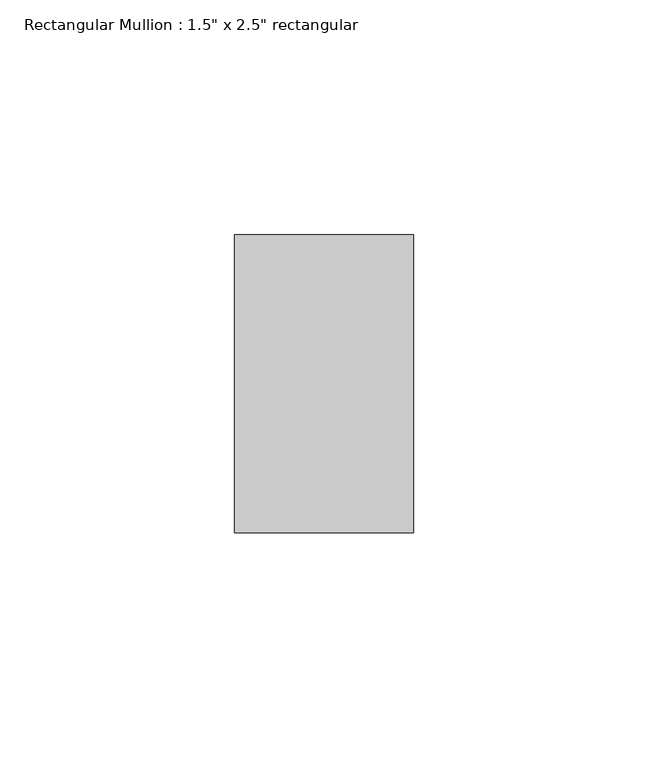
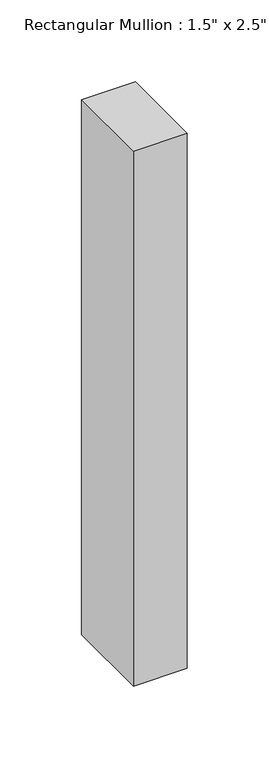
"""IFC4 building model written with IfcOpenShell, lengths in millimetres: member geometry."""

from ifc_helpers import new_model, si_unit, frame, origin, place, context, project, spatial, polyline, outline, extrude, source, transform, mapped, element, save


def member_20da7b42(model_context):
    return source(origin(), model_context, "Body", "SweptSolid", [
        extrude(outline(polyline([(0.0, 31.75), (0.0, -31.75), (-38.1, -31.75), (-38.1, 31.75), (0.0, 31.75)])), frame((0.0, 0.0, -400.05), z_axis=(0.0, 0.0, 1.0), x_axis=(1.0, 0.0, 0.0)), (0.0, 0.0, 1.0), 400.05),
    ])


if __name__ == "__main__":
    model = new_model("IFC4")
    model_context = context("Model", 3, world=origin())
    ifc_project = project(units=[si_unit("LENGTHUNIT", "METRE", prefix="MILLI")], contexts=[model_context])
    site = spatial("IfcSite", under=ifc_project)
    building = spatial("IfcBuilding", under=site)
    placement = place(None, origin())
    member_shape = member_20da7b42(model_context)
    element("IfcMember", 1, ObjectType="Rectangular Mullion : 1.5\" x 2.5\" rectangular", at=placement, inside=building, context=model_context, shape_type="MappedRepresentation", body=[
        mapped(member_shape, transform((0.0, 0.0, 0.0), x_axis=(1.0, 0.0, 0.0), y_axis=(0.0, 1.0, 0.0), z_axis=(0.0, 0.0, 1.0))),
    ])
    save(model, "model.ifc")

# Revit data of these elements
# Type "Rectangular Mullion : 1.5\" x 2.5\" rectangular"
#   built-in parameter 1007304 = 0.208333 (stored number, unit not read)
#   built-in parameter 1007301 = 0.0625 (stored number, unit not read)
#   built-in parameter 1007300 = 0.0625 (stored number, unit not read)
# Element 1 (IfcMember, "Rectangular Mullion : 1.5\" x 2.5\" rectangular")
#   Materials on its faces: "Aluminum"
# Materials
#   "Aluminum": class "Metal", colour RGB 247 247 247, transparency 0, Description = "Aluminum 6061", Cost = 0
